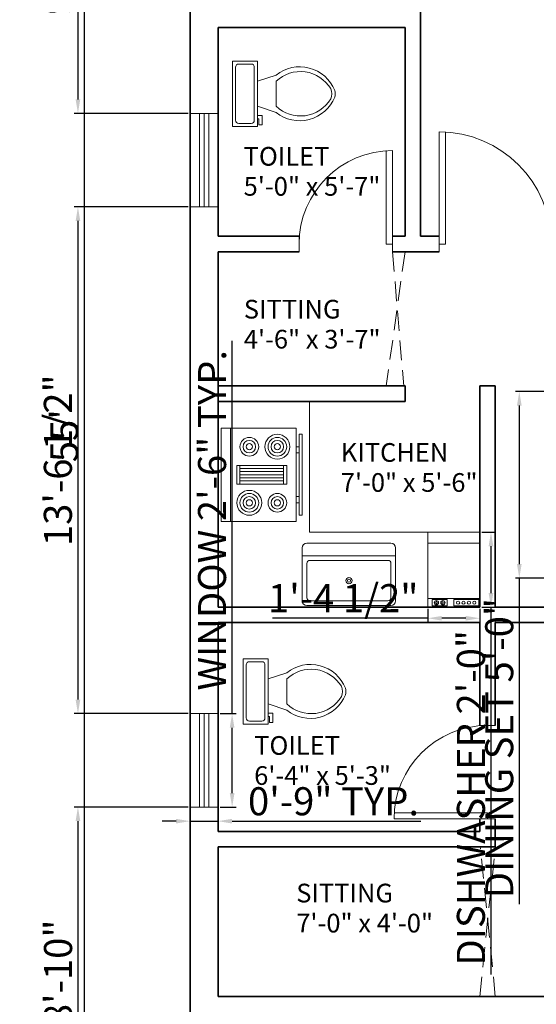
# Model space of a CAD drawing. Units: inches. Extents: x 3087 to 8148, y 1377 to 3709.
# Tile 2 of 6: x 3105 to 3271, y 1561 to 1877. Entities that reach past the tile are written whole.
import ezdxf

# ---------------------------------------------------------------- set-up
doc = ezdxf.new("R2010")
doc.units = ezdxf.units.IN
doc.linetypes.add('HIDDEN', pattern=[9.525, 6.35, -3.175])
for name, color, linetype, lineweight, true_color in [('A-ANNO-DIMS', 244, 'Continuous', 18, 0x991b1e), ('A-AREA-IDEN', 244, 'Continuous', 18, 0x991b1e), ('A-DOOR', 146, 'Continuous', 18, 0x105689), ('A-GLAZ', 146, 'Continuous', 18, 0x105689), ('A-WALL', 241, 'Continuous', 35, 0xf7abae), ('A-WALL-HIDN', 244, 'HIDDEN', 13, 0x991b1e)]:
    doc.layers.add(name, color=color, linetype=linetype, lineweight=lineweight, true_color=true_color)
for name, color, linetype, lineweight in [('A-EQPM', 8, 'Continuous', 18), ('A-FLOR-CASE', 9, 'Continuous', 18), ('A-FLOR-FIXT', 9, 'Continuous', 18)]:
    doc.layers.add(name, color=color, linetype=linetype, lineweight=lineweight)
doc.styles.get("Standard").update_dxf_attribs({"font": 'arial.ttf'})
doc.dimstyles.new('ISO-25', dxfattribs={"dimtxt": 9, "dimasz": 4.5, "dimexe": 1.25, "dimexo": 0.625, "dimtad": 1, "dimdec": 0, "dimlunit": 3, "dimtxsty": 'Standard', "dimcen": 2.5, "dimadec": 0, "dimazin": 0, "dimtfac": 1, "dimtdec": 0, "dimtmove": 0, "dimatfit": 3, "dimfxl": 1, "dimarcsym": 0})

# ---------------------------------------------------------------- blocks, each defined once
blk = doc.blocks.new('Toilet - top')
for p, q in [((9.5, -6), (9.5, -2)), ((-10, -8.5), (-8, -8.5)), ((-10, -9.5), (-10, -8.5)), ((-8, -8.5), (-8, -8)), ((-7, -8), (-7, -9.5)), ((-4, -8), (-6, -14)), ((4, -8), (6, -14)), ((-7, -9.5), (-10, -9.5)), ((4, -14), (-4, -14))]:
    blk.add_line(p, q)
blk.add_lwpolyline([(10.5, -8), (10.5, 0), (-10.5, 0), (-10.5, -8)], close=True)
for points in [[(-9.5, -2), (-9.5, -6)], [(8.5, -1), (-8.5, -1)], [(-8.5, -7), (8.5, -7)]]:
    blk.add_lwpolyline(points)
for centre, radius, start, end in [((-8.62, -1.88), 0.884, 81.8699, 188.1301), ((8.62, -1.88), 0.884, 351.8699, 98.1301), ((-8.62, -6.12), 0.884, 171.8699, 278.1301), ((8.62, -6.12), 0.884, 261.8699, 8.1301), ((3.52, -21.58), 12.17, 141.4691, 247.9714), ((4.2, -21.82), 11.33, 136.3677, 238.9468), ((-3.52, -21.58), 12.17, 292.0284, 38.5307), ((-4.2, -21.82), 11.33, 301.053, 43.6321), ((0, -27.88), 4, 245.7318, 294.2682), ((0, -29), 4, 254.8605, 285.1395)]:
    blk.add_arc(centre, radius, start, end)
blk = doc.blocks.new('Range-Oven - 30 in top')
for p, q in [((0, -3), (30, -3)), ((12, -6), (18, -6)), ((13, -20), (13, -6)), ((14, -6), (14, -20)), ((15, -20), (15, -6)), ((16, -6), (16, -20)), ((17, -20), (17, -6)), ((18, -20), (12, -20)), ((6, -24), (6, -25)), ((8, -25), (8, -24)), ((22, -25), (22, -24)), ((24, -24), (24, -25))]:
    blk.add_line(p, q)
for points in [[(0, -24), (0, 0), (30, 0), (30, -24)], [(12, -21), (12, -5), (18, -5), (18, -21)], [(2, -26), (2, -25), (28, -25), (28, -26)]]:
    blk.add_lwpolyline(points, close=True)
for centre, radius in [((6, -9), 4), ((6, -9), 3), ((24, -9), 3), ((6, -9), 2), ((6, -9), 1), ((24, -9), 2), ((24, -9), 1), ((6, -18), 3), ((24, -18), 4), ((24, -18), 3), ((6, -18), 2), ((6, -18), 1), ((24, -18), 2), ((24, -18), 1)]:
    blk.add_circle(centre, radius)
blk = doc.blocks.new('Sink-single - 30 in top')
blk.add_line((-15, -3.999996), (15, -3.999996))
for points in [[(-13.5, 0), (13.5, 0)], [(-15, -18.499996), (-15, -1.5)], [(15, -1.5), (15, -18.499996)], [(-12.5, -5.499996), (12.5, -5.499996)], [(-13.5, -17.499996), (-13.5, -6.499996)], [(13.5, -6.499996), (13.5, -17.499996)], [(12.5, -18.499996), (-12.5, -18.499996)], [(13.5, -19.999996), (-13.5, -19.999996)]]:
    blk.add_lwpolyline(points)
for radius in [1, 0.5]:
    blk.add_circle((0, -11.999996), radius)
for centre, radius, start, end in [((-13.5, -1.5), 1.5, 90, 180), ((13.5, -1.5), 1.5, 0, 90), ((-12.5, -6.499996), 1, 90, 180), ((12.5, -6.499996), 1, 0, 90), ((-13.5, -18.499996), 1.5, 180, 270), ((-12.5, -17.499996), 1, 180, 270), ((12.5, -17.499996), 1, 270, 0), ((13.5, -18.499996), 1.5, 270, 0)]:
    blk.add_arc(centre, radius, start, end)
blk = doc.blocks.new('Dishwasher')
for p, q in [((16, 32.5), (16.75, 32.5)), ((16.5, 32), (16.2942, 31.7942)), ((16.3156, 33.1843), (16.5, 33)), ((17, 32.75), (17, 33.5)), ((17, 32.25), (17, 31.5)), ((18, 32.5), (17.25, 32.5)), ((17.5, 33), (17.6938, 33.1938)), ((17.7061, 31.7939), (17.5, 32)), ((19, 32.5), (19.75, 32.5)), ((19.5, 32), (19.2942, 31.7942)), ((19.3156, 33.1843), (19.5, 33)), ((20, 32.75), (20, 33.5)), ((20, 32.25), (20, 31.5)), ((21, 32.5), (20.25, 32.5)), ((20.5, 33), (20.6938, 33.1938)), ((20.7061, 31.7939), (20.5, 32)), ((24, 30.5), (0, 30.5)), ((0, 5), (24, 5))]:
    blk.add_line(p, q)
for points in [[(0, 0), (0, 34.5), (24, 34.5), (24, 0)], [(0.5, 31), (0.5, 34), (12, 34), (12, 31)], [(15, 31), (15, 34), (22, 34), (22, 31)]]:
    blk.add_lwpolyline(points, close=True)
for centre, radius in [((2.5, 32.5), 0.75), ((5, 32.5), 0.75), ((7.5, 32.5), 0.75), ((10, 32.5), 0.75), ((17, 32.5), 1), ((20, 32.5), 1)]:
    blk.add_circle(centre, radius)
blk = doc.blocks.new('*D18')
at = {"layer": 'A-ANNO-DIMS', "color": 0, "lineweight": -2, "transparency": 16777216}
for p, q in [((3159.19, 2073.96), (3124.53, 2073.96)), ((3125.78, 2069.46), (3125.78, 1418.46)), ((3159.19, 1413.96), (3124.53, 1413.96))]:
    blk.add_line(p, q, dxfattribs=at)
at = {"layer": 'A-ANNO-DIMS', "color": 0, "transparency": 16777216}
for points in [[(3125.03, 2069.46), (3126.53, 2069.46), (3125.78, 2073.96)], [(3125.03, 1418.46), (3126.53, 1418.46), (3125.78, 1413.96)]]:
    blk.add_solid(points, dxfattribs=at)
at = {"layer": 'Defpoints', "color": 0, "transparency": 16777216}
for p in [(3159.82, 2073.96), (3125.78, 1413.96), (3159.82, 1413.96)]:
    blk.add_point(p, dxfattribs=at)
at = {"layer": 'A-ANNO-DIMS', "color": 0, "transparency": 16777216, "insert": (3120.58, 1743.96), "char_height": 9, "attachment_point": 5, "rotation": 90}
blk.add_mtext("55'", dxfattribs=at)
blk = doc.blocks.new('DOOR-SINGLE-30IN')
for p, q in [((0, 30), (30, 30)), ((30, 30), (30, 28)), ((0, 28), (30, 28))]:
    blk.add_line(p, q)
blk.add_arc((30, 30), 30, 180, 270)
blk = doc.blocks.new('DOOR-SINGLE-36IN')
for p, q in [((0, 2), (36, 2)), ((36, 0), (36, 2)), ((0, 0), (36, 0))]:
    blk.add_line(p, q)
blk.add_arc((36, 0), 36, 90, 180)
blk = doc.blocks.new('WINDOW-30IN')
for p, q in [((0, 0), (0, 30)), ((9, 30), (0, 30)), ((3, 30), (3, 0)), ((4.5, 30), (4.5, 0)), ((6, 30), (6, 0)), ((9, 30), (9, 0)), ((9, 0), (0, 0))]:
    blk.add_line(p, q)
blk = doc.blocks.new('*D37')
at = {"layer": 'A-ANNO-DIMS', "color": 0, "lineweight": -2, "transparency": 16777216}
for p, q in [((3173.32, 1654.74), (3173.32, 1774.38)), ((3169.44, 1654.74), (3174.57, 1654.74)), ((3173.32, 1629.24), (3173.32, 1650.24)), ((3169.44, 1624.74), (3174.57, 1624.74))]:
    blk.add_line(p, q, dxfattribs=at)
at = {"layer": 'A-ANNO-DIMS', "color": 0, "transparency": 16777216}
for points in [[(3172.57, 1650.24), (3174.07, 1650.24), (3173.32, 1654.74)], [(3172.57, 1629.24), (3174.07, 1629.24), (3173.32, 1624.74)]]:
    blk.add_solid(points, dxfattribs=at)
at = {"layer": 'Defpoints', "color": 0, "transparency": 16777216}
for p in [(3168.82, 1654.74), (3173.32, 1654.74), (3168.82, 1624.74)]:
    blk.add_point(p, dxfattribs=at)
at = {"layer": 'A-ANNO-DIMS', "color": 0, "transparency": 16777216, "insert": (3168.04, 1716.81), "char_height": 9, "attachment_point": 5, "rotation": 90}
blk.add_mtext('WINDOW 2\'-6" TYP.', dxfattribs=at)
blk = doc.blocks.new('*D38')
at = {"layer": 'A-ANNO-DIMS', "color": 0, "lineweight": -2, "transparency": 16777216}
for p, q in [((3159.82, 1624.12), (3159.82, 1618.99)), ((3168.82, 1624.12), (3168.82, 1618.99)), ((3155.32, 1620.24), (3150.82, 1620.24)), ((3159.82, 1620.24), (3168.82, 1620.24)), ((3173.32, 1620.24), (3233.93, 1620.24))]:
    blk.add_line(p, q, dxfattribs=at)
at = {"layer": 'A-ANNO-DIMS', "color": 0, "transparency": 16777216}
for points in [[(3155.32, 1620.99), (3155.32, 1619.49), (3159.82, 1620.24)], [(3173.32, 1620.99), (3173.32, 1619.49), (3168.82, 1620.24)]]:
    blk.add_solid(points, dxfattribs=at)
at = {"layer": 'Defpoints', "color": 0, "transparency": 16777216}
for p in [(3159.82, 1624.74), (3168.82, 1624.74), (3168.82, 1620.24)]:
    blk.add_point(p, dxfattribs=at)
at = {"layer": 'A-ANNO-DIMS', "color": 0, "transparency": 16777216, "insert": (3205.87, 1625.46), "char_height": 9, "attachment_point": 5}
blk.add_mtext('0\'-9" TYP.', dxfattribs=at)
blk = doc.blocks.new('*D43')
at = {"layer": 'A-ANNO-DIMS', "color": 0, "lineweight": -2, "transparency": 16777216}
for p, q in [((3273.87, 1758.14), (3264.27, 1758.14)), ((3265.52, 1753.64), (3265.52, 1702.76)), ((3273.87, 1698.26), (3264.27, 1698.26)), ((3265.52, 1698.26), (3265.52, 1593.59))]:
    blk.add_line(p, q, dxfattribs=at)
at = {"layer": 'A-ANNO-DIMS', "color": 0, "transparency": 16777216}
for points in [[(3264.77, 1753.64), (3266.27, 1753.64), (3265.52, 1758.14)], [(3264.77, 1702.76), (3266.27, 1702.76), (3265.52, 1698.26)]]:
    blk.add_solid(points, dxfattribs=at)
at = {"layer": 'Defpoints', "color": 0, "transparency": 16777216}
for p in [(3274.5, 1758.14), (3265.52, 1698.26), (3274.5, 1698.26)]:
    blk.add_point(p, dxfattribs=at)
at = {"layer": 'A-ANNO-DIMS', "color": 0, "transparency": 16777216, "insert": (3260.24, 1643.68), "char_height": 9, "attachment_point": 5, "rotation": 90}
blk.add_mtext('DINING SET 5\'-0"', dxfattribs=at)
blk = doc.blocks.new('*D57')
at = {"layer": 'A-ANNO-DIMS', "color": 0, "lineweight": -2, "transparency": 16777216}
for p, q in [((3253.44, 1712.96), (3257.67, 1712.96)), ((3256.42, 1708.46), (3256.42, 1693.46)), ((3253.44, 1688.96), (3257.67, 1688.96)), ((3256.42, 1688.96), (3256.42, 1571.02))]:
    blk.add_line(p, q, dxfattribs=at)
at = {"layer": 'A-ANNO-DIMS', "color": 0, "transparency": 16777216}
for points in [[(3255.67, 1708.46), (3257.17, 1708.46), (3256.42, 1712.96)], [(3255.67, 1693.46), (3257.17, 1693.46), (3256.42, 1688.96)]]:
    blk.add_solid(points, dxfattribs=at)
at = {"layer": 'Defpoints', "color": 0, "transparency": 16777216}
for p in [(3252.82, 1712.96), (3252.82, 1688.96), (3256.42, 1688.96)]:
    blk.add_point(p, dxfattribs=at)
at = {"layer": 'A-ANNO-DIMS', "color": 0, "transparency": 16777216, "insert": (3251.14, 1627.74), "char_height": 9, "attachment_point": 5, "rotation": 90}
blk.add_mtext('DISHWASHER 2\'-0"', dxfattribs=at)
blk = doc.blocks.new('*D58')
at = {"layer": 'A-ANNO-DIMS', "color": 0, "lineweight": -2, "transparency": 16777216}
for p, q in [((3236.12, 1688.34), (3236.12, 1684.11)), ((3252.82, 1688.34), (3252.82, 1684.11)), ((3236.12, 1685.36), (3186.32, 1685.36)), ((3248.32, 1685.36), (3240.62, 1685.36))]:
    blk.add_line(p, q, dxfattribs=at)
at = {"layer": 'A-ANNO-DIMS', "color": 0, "transparency": 16777216}
for points in [[(3240.62, 1686.11), (3240.62, 1684.61), (3236.12, 1685.36)], [(3248.32, 1686.11), (3248.32, 1684.61), (3252.82, 1685.36)]]:
    blk.add_solid(points, dxfattribs=at)
at = {"layer": 'Defpoints', "color": 0, "transparency": 16777216}
for p in [(3236.12, 1688.96), (3252.82, 1688.96), (3236.12, 1685.36)]:
    blk.add_point(p, dxfattribs=at)
at = {"layer": 'A-ANNO-DIMS', "color": 0, "transparency": 16777216, "insert": (3208.97, 1690.64), "char_height": 9, "attachment_point": 5}
blk.add_mtext('1\'-4 1/2"', dxfattribs=at)
blk = doc.blocks.new('*D62')
at = {"layer": 'A-ANNO-DIMS', "color": 0, "lineweight": -2, "transparency": 16777216}
for p, q in [((3159.19, 1966.01), (3122.57, 1966.01)), ((3123.82, 1961.51), (3123.82, 1851.89)), ((3159.19, 1847.39), (3122.57, 1847.39))]:
    blk.add_line(p, q, dxfattribs=at)
at = {"layer": 'A-ANNO-DIMS', "color": 0, "transparency": 16777216}
for points in [[(3123.07, 1961.51), (3124.57, 1961.51), (3123.82, 1966.01)], [(3123.07, 1851.89), (3124.57, 1851.89), (3123.82, 1847.39)]]:
    blk.add_solid(points, dxfattribs=at)
at = {"layer": 'Defpoints', "color": 0, "transparency": 16777216}
for p in [(3159.82, 1966.01), (3123.82, 1847.39), (3159.82, 1847.39)]:
    blk.add_point(p, dxfattribs=at)
at = {"layer": 'A-ANNO-DIMS', "color": 0, "transparency": 16777216, "insert": (3118.54, 1906.7), "char_height": 9, "attachment_point": 5, "rotation": 90}
blk.add_mtext('9\'-10 1/2"', dxfattribs=at)
blk = doc.blocks.new('*D63')
at = {"layer": 'A-ANNO-DIMS', "color": 0, "lineweight": -2, "transparency": 16777216}
for p, q in [((3159.19, 1817.39), (3122.57, 1817.39)), ((3123.82, 1812.89), (3123.82, 1659.24)), ((3159.19, 1654.74), (3122.57, 1654.74))]:
    blk.add_line(p, q, dxfattribs=at)
at = {"layer": 'A-ANNO-DIMS', "color": 0, "transparency": 16777216}
for points in [[(3123.07, 1812.89), (3124.57, 1812.89), (3123.82, 1817.39)], [(3123.07, 1659.24), (3124.57, 1659.24), (3123.82, 1654.74)]]:
    blk.add_solid(points, dxfattribs=at)
at = {"layer": 'Defpoints', "color": 0, "transparency": 16777216}
for p in [(3159.82, 1817.39), (3123.82, 1654.74), (3159.82, 1654.74)]:
    blk.add_point(p, dxfattribs=at)
at = {"layer": 'A-ANNO-DIMS', "color": 0, "transparency": 16777216, "insert": (3118.54, 1736.07), "char_height": 9, "attachment_point": 5, "rotation": 90}
blk.add_mtext('13\'-6 1/2"', dxfattribs=at)
blk = doc.blocks.new('*D64')
at = {"layer": 'A-ANNO-DIMS', "color": 0, "lineweight": -2, "transparency": 16777216}
for p, q in [((3159.19, 1624.74), (3122.57, 1624.74)), ((3123.82, 1620.24), (3123.82, 1523.18)), ((3159.19, 1518.68), (3122.57, 1518.68))]:
    blk.add_line(p, q, dxfattribs=at)
at = {"layer": 'A-ANNO-DIMS', "color": 0, "transparency": 16777216}
for points in [[(3123.07, 1620.24), (3124.57, 1620.24), (3123.82, 1624.74)], [(3123.07, 1523.18), (3124.57, 1523.18), (3123.82, 1518.68)]]:
    blk.add_solid(points, dxfattribs=at)
at = {"layer": 'Defpoints', "color": 0, "transparency": 16777216}
for p in [(3159.82, 1624.74), (3123.82, 1518.68), (3159.82, 1518.68)]:
    blk.add_point(p, dxfattribs=at)
at = {"layer": 'A-ANNO-DIMS', "color": 0, "transparency": 16777216, "insert": (3118.6, 1571.71), "char_height": 9, "attachment_point": 5, "rotation": 90}
blk.add_mtext('8\'-10"', dxfattribs=at)

msp = doc.modelspace()

# ---------------------------------------------------------------- linework, layer by layer
at = {"layer": 'A-DOOR'}
for p, q in [((3194.82, 1802.96), (3194.82, 1807.96)), ((3224.82, 1802.96), (3224.82, 1807.96)), ((3239.82, 1802.96), (3239.82, 1807.96)), ((3252.82, 1650.96), (3257.82, 1650.96)), ((3252.82, 1620.96), (3257.82, 1620.96))]:
    msp.add_line(p, q, dxfattribs=at)
at = {"layer": 'A-FLOR-CASE'}
for p, q in [((3198.14, 1712.96), (3198.14, 1754.96)), ((3252.82, 1712.96), (3198.14, 1712.96))]:
    msp.add_line(p, q, dxfattribs=at)
at = {"layer": 'A-WALL'}
for p, q in [((3159.82, 1413.96), (3159.82, 2073.96)), ((3233.82, 1807.96), (3233.82, 1879.96)), ((3168.82, 1874.96), (3228.82, 1874.96)), ((3168.82, 1807.96), (3168.82, 1874.96)), ((3228.82, 1807.96), (3228.82, 1874.96)), ((3168.82, 1807.96), (3194.82, 1807.96)), ((3224.82, 1807.96), (3228.82, 1807.96)), ((3233.82, 1807.96), (3239.82, 1807.96)), ((3168.82, 1802.96), (3194.82, 1802.96)), ((3168.82, 1688.96), (3168.82, 1802.96)), ((3224.82, 1802.96), (3239.82, 1802.96)), ((3168.82, 1759.96), (3228.82, 1759.96)), ((3228.82, 1754.96), (3228.82, 1759.96)), ((3252.82, 1759.96), (3257.82, 1759.96)), ((3252.82, 1688.96), (3252.82, 1759.96)), ((3257.82, 1688.96), (3257.82, 1759.96)), ((3168.82, 1754.96), (3228.82, 1754.96)), ((3168.82, 1688.96), (3252.82, 1688.96)), ((3257.82, 1688.96), (3335.82, 1688.96)), ((3168.82, 1683.96), (3252.82, 1683.96)), ((3168.82, 1616.96), (3168.82, 1683.96)), ((3252.82, 1650.96), (3252.82, 1683.96)), ((3257.82, 1650.96), (3257.82, 1683.96)), ((3257.82, 1683.96), (3335.82, 1683.96)), ((3252.82, 1616.96), (3252.82, 1620.96)), ((3257.82, 1611.96), (3257.82, 1620.96)), ((3168.82, 1616.96), (3252.82, 1616.96)), ((3168.82, 1611.96), (3257.82, 1611.96)), ((3168.82, 1563.96), (3168.82, 1611.96)), ((3168.82, 1563.96), (3257.82, 1563.96)), ((3257.82, 1563.96), (3377.82, 1563.96))]:
    msp.add_line(p, q, dxfattribs=at)
at = {"layer": 'A-WALL-HIDN'}
for p, q in [((3228.82, 1802.96), (3222.82, 1759.96)), ((3224.82, 1802.96), (3228.4, 1759.96)), ((3252.82, 1563.96), (3257.82, 1611.96)), ((3257.82, 1563.96), (3252.96, 1611.96))]:
    msp.add_line(p, q, dxfattribs=at)

# ---------------------------------------------------------------- block references
at = {"layer": 'A-DOOR'}
for name, p, rotation in [('DOOR-SINGLE-36IN', (3239.82, 1841.46), 270.0000000000006), ('DOOR-SINGLE-30IN', (3194.82, 1835.46), 269.999999999999)]:
    msp.add_blockref(name, p, dxfattribs=dict(at, rotation=rotation))
at = {"layer": 'A-DOOR', "extrusion": (0, 0, -1), "zscale": -1, "rotation": 180}
msp.add_blockref('DOOR-SINGLE-30IN', (-3225.32, 1650.96), dxfattribs=at)
at = {"layer": 'A-EQPM', "rotation": 90}
msp.add_blockref('Range-Oven - 30 in top', (3169.84, 1716.41), dxfattribs=at)
at = {"layer": 'A-EQPM', "xscale": 0.6956521739130344, "yscale": 0.6956521739130344, "zscale": 0.6956521739130344, "rotation": 180.0000000000009}
msp.add_blockref('Dishwasher', (3252.82, 1712.96), dxfattribs=at)
at = {"layer": 'A-FLOR-FIXT', "rotation": 90}
for p in [(3173.43, 1853.68), (3176.87, 1661.87)]:
    msp.add_blockref('Toilet - top', p, dxfattribs=at)
at = {"layer": 'A-FLOR-FIXT'}
msp.add_blockref('Sink-single - 30 in top', (3210.82, 1709.44), dxfattribs=at)
at = {"layer": 'A-GLAZ'}
for p in [(3159.82, 1817.39), (3159.82, 1624.74)]:
    msp.add_blockref('WINDOW-30IN', p, dxfattribs=at)

# ---------------------------------------------------------------- texts
at = {"layer": 'A-AREA-IDEN'}
for s, p in [('TOILET ', (3177.02, 1830.61)), ('5\'-0" x 5\'-7"', (3177.02, 1820.97)), ('SITTING', (3177.07, 1781.55)), ('4\'-6" x 3\'-7"', (3177.07, 1771.92)), ('KITCHEN', (3208.21, 1735.57)), ('7\'-0" x 5\'-6"', (3208.21, 1725.93)), ('TOILET', (3180.4, 1641.53)), ('6\'-4" x 5\'-3"', (3180.4, 1631.89)), ('SITTING', (3193.91, 1594.16)), ('7\'-0" x 4\'-0"', (3193.91, 1584.52))]:
    msp.add_text(s, height=6, dxfattribs=at).set_placement(p)

# ---------------------------------------------------------------- dimensions: what is measured, and where the dimension line sits
at = {"layer": 'A-ANNO-DIMS'}
for base, p1, p2, angle, override, picture, middle in [((3125.78, 1413.96), (3159.82, 2073.96), (3159.82, 1413.96), 90, {"dimclrd": 0, "dimclre": 0, "dimclrt": 0}, '*D18', (3120.58, 1743.96)), ((3123.82, 1847.39), (3159.82, 1966.01), (3159.82, 1847.39), 90, {"dimdec": 1, "dimlfac": 1, "dimrnd": 0, "dimzin": 1, "dimdsep": 46, "dimlunit": 4, "dimfrac": 2}, '*D62', (3118.54, 1906.7)), ((3123.8176, 1654.7438), (3159.8176, 1817.3887), (3159.8176, 1654.7438), 90, {"dimdec": 1, "dimlfac": 1, "dimrnd": 0, "dimzin": 1, "dimdsep": 46, "dimlunit": 4, "dimfrac": 2}, '*D63', (3118.536, 1736.0663)), ((3236.12, 1685.36), (3252.82, 1688.96), (3236.12, 1688.96), 180, {"dimdec": 1, "dimlfac": 1, "dimrnd": 0, "dimzin": 1, "dimdsep": 46, "dimlunit": 4, "dimfrac": 2}, '*D58', (3208.97, 1690.64)), ((3123.82, 1518.68), (3159.82, 1624.74), (3159.82, 1518.68), 90, {"dimdec": 1, "dimlfac": 1, "dimrnd": 0, "dimzin": 1, "dimdsep": 46, "dimlunit": 4, "dimfrac": 2}, '*D64', (3118.6, 1571.71))]:
    dim = msp.add_linear_dim(base=base, p1=p1, p2=p2, angle=angle, dimstyle='ISO-25', override=override, dxfattribs=at)
    dim.commit()
    dim.dimension.update_dxf_attribs({"geometry": picture, "text_midpoint": middle})
for base, p1, p2, angle, text, picture, middle in [((3173.32, 1654.74), (3168.82, 1624.74), (3168.82, 1654.74), 90, 'WINDOW <> TYP.', '*D37', (3168.04, 1716.81)), ((3265.52, 1698.26), (3274.5, 1758.14), (3274.5, 1698.26), 270, 'DINING SET <>', '*D43', (3260.24, 1643.68)), ((3256.42, 1688.96), (3252.82, 1712.96), (3252.82, 1688.96), 270, 'DISHWASHER <>', '*D57', (3251.14, 1627.74))]:
    dim = msp.add_linear_dim(base=base, p1=p1, p2=p2, angle=angle, text=text, dimstyle='ISO-25', override={"dimdec": 1, "dimlfac": 1, "dimrnd": 0, "dimzin": 1, "dimdsep": 46, "dimlunit": 4, "dimfrac": 2}, dxfattribs=at)
    dim.commit()
    dim.dimension.update_dxf_attribs({"geometry": picture, "text_midpoint": middle})
dim = msp.add_linear_dim(base=(3168.82, 1620.24), p1=(3159.82, 1624.74), p2=(3168.82, 1624.74), text='<> TYP.', dimstyle='ISO-25', override={"dimdec": 1, "dimlfac": 1, "dimrnd": 0, "dimzin": 1, "dimdsep": 46, "dimlunit": 4, "dimfrac": 2}, dxfattribs=at)
dim.commit()
dim.dimension.update_dxf_attribs({"geometry": '*D38', "text_midpoint": (3205.87, 1625.46)})

doc.saveas('drawing.dxf')
